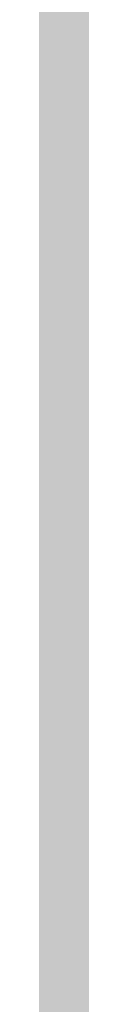
# Model space of a CAD drawing. Units: inches. Extents: x 2083 to 3317, y 1141 to 2115.
# Tile 169 of 256: x 3126.959398 to 3126.959687, y 1263.265937 to 1263.274018. Entities that reach past the tile are written whole.
import ezdxf

# ---------------------------------------------------------------- set-up
doc = ezdxf.new("R2010")
doc.units = ezdxf.units.IN
doc.layers.add('A-ANNO-DIMS', color=2, linetype='Continuous', lineweight=18)
doc.layers.add('A-WALL-PATT', color=251, linetype='Continuous', lineweight=13, true_color=0x636466)
doc.styles.get("Standard").update_dxf_attribs({"font": 'arial.ttf'})
doc.dimstyles.new('ISO-25', dxfattribs={"dimtxt": 12, "dimasz": 12, "dimexe": 1.25, "dimexo": 0.625, "dimtad": 1, "dimlunit": 3, "dimtxsty": 'Standard', "dimcen": 2.5, "dimadec": 0, "dimazin": 0, "dimtfac": 1, "dimtmove": 0, "dimatfit": 3, "dimfxl": 1, "dimarcsym": 0})

# ---------------------------------------------------------------- blocks, each defined once
blk = doc.blocks.new('*D26')
at = {"layer": 'A-ANNO-DIMS', "color": 0, "lineweight": -2, "transparency": 16777216}
for p, q in [((3088.985844, 1274.915092), (3088.985844, 1270.9519631)), ((3111.2400366, 1274.915092), (3111.2400366, 1270.9519631)), ((3076.985844, 1272.2019631), (2840.262447, 1272.2019631)), ((3111.2400366, 1272.2019631), (3088.985844, 1272.2019631)), ((3123.2400366, 1272.2019631), (3135.2400366, 1272.2019631))]:
    blk.add_line(p, q, dxfattribs=at)
at = {"layer": 'A-ANNO-DIMS', "color": 0, "transparency": 16777216}
for points in [[(3076.985844, 1274.2019631), (3076.985844, 1270.2019631), (3088.985844, 1272.2019631)], [(3123.2400366, 1274.2019631), (3123.2400366, 1270.2019631), (3111.2400366, 1272.2019631)]]:
    blk.add_solid(points, dxfattribs=at)
at = {"layer": 'Defpoints', "color": 0, "transparency": 16777216}
for p in [(3088.985844, 1275.540092), (3111.2400366, 1275.540092), (3088.985844, 1272.2019631)]:
    blk.add_point(p, dxfattribs=at)
at = {"layer": 'A-ANNO-DIMS', "color": 0, "transparency": 16777216, "insert": (2952.6241455, 1279.0316016), "char_height": 12, "attachment_point": 5}
blk.add_mtext('NIGHTSTAND 1\'-10 1/2" TYP.', dxfattribs=at)

msp = doc.modelspace()

# ---------------------------------------------------------------- hatches: boundary and pattern name
at = {"layer": 'A-WALL-PATT'}
h = msp.add_hatch(color=256, dxfattribs=at)
h.dxf.hatch_style = 1
h.paths.add_polyline_path([(3126.9597832, 2020.7613601), (2748.9597832, 2020.7613601), (2604.9597832, 2020.7613601), (2226.9597832, 2020.7613601), (2226.9597832, 1702.7613601), (2466.9597832, 1702.7613601), (2466.9597832, 1582.7613601), (2418.9597832, 1582.7613601), (2418.9597832, 1477.7613601), (2226.9597832, 1477.7613601), (2226.9597832, 1263.2613601), (2544.9597832, 1263.2613601), (2544.9597832, 1411.7613601), (2604.9597832, 1411.7613601), (2685.9597832, 1411.7613601), (2685.9597832, 1420.7613601), (2604.9597832, 1420.7613601), (2604.9597832, 1573.7613601), (2604.9597832, 1702.7613601), (2604.9597832, 2011.7613601), (2748.9597832, 2011.7613601), (2748.9597832, 1702.7613601), (2862.9597832, 1702.7613601), (2862.9597832, 1621.7613601), (2871.9597832, 1621.7613601), (2871.9597832, 1702.7613601), (2883.9597832, 1702.7613601), (2883.9597832, 1706.9394595, -0.026459), (2883.9597832, 1711.7613601), (2757.9597832, 1711.7613601), (2757.9597832, 1807.7613601), (2787.9597832, 1807.7613601), (2787.9597832, 1812.2613601), (2757.9597832, 1812.2613601), (2757.9597832, 2011.7613601), (2877.9597832, 2011.7613601), (2877.9597832, 1812.2613601), (2847.9597832, 1812.2613601), (2847.9597832, 1807.7613601), (2889.8357425, 1807.7613601), (2889.8357425, 1812.2613601), (2882.4597832, 1812.2613601), (2882.4597832, 2011.7613601), (3117.9597832, 2011.7613601), (3117.9597832, 1812.2613601), (2937.8357425, 1812.2613601), (2937.8357425, 1807.7613601), (2995.7097832, 1807.7613601), (2995.7097832, 1796.1176655), (3000.2097832, 1796.1176655), (3000.2097832, 1807.7613601), (3117.9597832, 1807.7613601), (3117.9597832, 1711.7613601), (3000.2097832, 1711.7613601), (3000.2097832, 1760.1176655), (2998.5727047, 1760.1176655, -0.020711), (2995.7097832, 1760.1176655), (2995.7097832, 1711.7613601), (2931.9597832, 1711.7613601), (2931.9597832, 1702.7613601), (3126.9597832, 1702.7613601)])
h.paths.add_polyline_path([(2471.4597832, 2011.7613601), (2471.4597832, 1810.0113601), (2462.7169357, 1810.0113601), (2462.7169357, 1805.5113601), (2505.9597832, 1805.5113601), (2505.9597832, 1810.0113601), (2475.9597832, 1810.0113601), (2475.9597832, 2011.7613601), (2595.9597832, 2011.7613601), (2595.9597832, 1810.0113601), (2565.9597832, 1810.0113601), (2565.9597832, 1805.5113601), (2595.9597832, 1805.5113601), (2595.9597832, 1711.7613601), (2235.9597832, 1711.7613601), (2235.9597832, 1805.5113601), (2353.7097832, 1805.5113601), (2353.7097832, 1796.0541624), (2358.2097832, 1796.0541624), (2358.2097832, 1805.5113601), (2414.7169357, 1805.5113601), (2414.7169357, 1810.0113601), (2235.9597832, 1810.0113601), (2235.9597832, 2011.7613601)], flags=16)
h.paths.add_polyline_path([(2270.2047343, 1994.6100082), (2270.2047343, 1970.6100082), (2246.2047343, 1970.6100082), (2246.2047343, 1994.6100082)], flags=0)
edge = h.paths.add_edge_path(flags=0)
edge.add_ellipse((2332.027391, 1899.7981761), major_axis=(-3.0429938, 3.0429938), ratio=0.16825245, start_angle=-161.3321656, end_angle=-156.3071136, ccw=False)
edge.add_ellipse((2333.0820373, 1898.7435297), major_axis=(-1.0546463, 1.0546463), ratio=0.453532097, start_angle=-123.371019, end_angle=-94.1591066)
edge = h.paths.add_edge_path(flags=0)
edge.add_ellipse((2332.027391, 1968.8762897), major_axis=(3.0429938, 3.0429938), ratio=0.16825245, start_angle=18.6678344, end_angle=23.6928864)
edge.add_spline(control_points=[(2332.9255964, 1970.6911045), (2332.2267681, 1970.3360997), (2330.8937087, 1969.6589054), (2328.4130803, 1970.9321376), (2327.2039345, 1967.7487119), (2324.7095965, 1969.9555886), (2322.5328223, 1967.012354), (2320.0128462, 1971.2958124), (2317.6803077, 1968.1578449), (2316.0405263, 1967.1020468), (2315.4269045, 1966.8096022)], knot_values=[0, 0, 0, 0, 2.267059, 4.324559, 6.685584, 8.878641, 11.121502, 14.300359, 17.755284, 19.732645, 19.732645, 19.732645, 19.732645], degree=3, periodic=0)
edge.add_ellipse((2332.027391, 1968.8762897), major_axis=(3.0429938, 3.0429938), ratio=0.16825245, start_angle=18.6678344, end_angle=23.6928864, ccw=False)
edge.add_ellipse((2333.0820373, 1969.930936), major_axis=(1.0546463, 1.0546463), ratio=0.453532097, start_angle=56.628981, end_angle=85.8408934, ccw=False)
edge = h.paths.add_edge_path(flags=0)
edge.add_spline(control_points=[(2296.4282874, 1967.9879081), (2293.6278045, 1965.3363137), (2287.7036238, 1959.727094), (2299.7438601, 1949.9956993), (2294.5325909, 1935.6685275), (2290.5732281, 1920.6035119), (2293.3941244, 1909.9736911), (2296.1854073, 1904.9665431)], knot_values=[0.099185, 0.099185, 0.099185, 0.099185, 0.345301, 0.619822, 0.982653, 1.386093, 1.810555, 1.810555, 1.810555, 1.810555], degree=3, periodic=0)
edge.add_spline(control_points=[(2296.1854073, 1904.9665431), (2297.3835817, 1902.6193002), (2298.0009694, 1901.9493116), (2298.5529698, 1901.4681549)], knot_values=[0.006246, 0.006246, 0.006246, 0.006246, 0.055476, 0.055476, 0.055476, 0.055476], degree=3, periodic=0)
edge.add_spline(control_points=[(2298.5529698, 1901.4681549), (2297.2586121, 1900.9232238), (2295.2252939, 1900.2321257), (2293.0602287, 1900.6142053), (2292.1014227, 1900.788415), (2292.0895776, 1900.790568)], knot_values=[0.312835, 0.312835, 0.312835, 0.312835, 0.40178, 0.474987, 0.475903, 0.475903, 0.475903, 0.475903], degree=3, periodic=0)
edge.add_arc((2292.7936464, 1904.6641088), 3.9370079, 215.4208969, 259.6981795, ccw=False)
edge.add_spline(control_points=[(2289.5853139, 1902.3823039), (2289.4766524, 1902.5350874), (2289.3684805, 1902.6880353), (2289.2608648, 1902.8411699)], knot_values=[0.102872, 0.102872, 0.102872, 0.102872, 0.116896, 0.116896, 0.116896, 0.116896], degree=3, periodic=0)
edge.add_spline(control_points=[(2289.2608648, 1902.8411699), (2288.6866042, 1902.5501922), (2287.6400477, 1902.0199025), (2285.8813368, 1901.8739536), (2283.8529717, 1901.5043521), (2281.7199871, 1899.7105375), (2278.4669913, 1899.492942), (2276.1571361, 1901.8832022), (2272.2589526, 1899.8040711), (2267.7776054, 1901.8431828), (2262.2438819, 1900.1840326), (2257.414927, 1901.7820606), (2254.318374, 1900.7261196), (2253.1782849, 1900.3373431)], knot_values=[0, 0, 0, 0, 1.907977, 3.477176, 5.261074, 7.972851, 11.680248, 13.717921, 16.939592, 22.789562, 27.502503, 33.595215, 37.145618, 37.145618, 37.145618, 37.145618], degree=3, periodic=0)
edge.add_line((2253.1782849, 1900.3373431), (2250.2442397, 1902.8411699))
edge.add_line((2250.2442397, 1902.8411699), (2250.2442397, 1965.8332959))
edge.add_line((2250.2442397, 1965.8332959), (2253.1782849, 1968.3371226))
edge.add_spline(control_points=[(2253.1782849, 1968.3371226), (2254.318374, 1967.9483462), (2257.414927, 1966.8924051), (2262.2438819, 1968.4904332), (2267.7776054, 1966.8312829), (2271.5267301, 1968.5372172), (2273.8759143, 1967.8282895), (2274.2067012, 1967.7276424)], knot_values=[0, 0, 0, 0, 0.09018, 0.244935, 0.364644, 0.513233, 0.537855, 0.537855, 0.537855, 0.537855], degree=3, periodic=0)
edge.add_arc((2274.3528869, 1963.7933495), 3.9370079, 72.0511336, 92.1279492, ccw=False)
edge.add_arc((2281.2969331, 1985.2300027), 18.5962982, 252.05113361, 288.56572166)
edge.add_arc((2292.3167172, 1956.0288805), 12.6460805, 71.02678788, 113.77821843, ccw=False)
edge = h.paths.add_edge_path(flags=0)
edge.add_spline(control_points=[(2274.8994147, 1951.8561946), (2275.066156, 1951.6165924), (2275.2326866, 1951.3765878), (2275.3979871, 1951.1358545)], knot_values=[1.409916, 1.409916, 1.409916, 1.409916, 1.43159, 1.43159, 1.43159, 1.43159], degree=3, periodic=0)
edge.add_spline(control_points=[(2275.3979871, 1951.1358545), (2275.7921055, 1950.5618854), (2276.1792311, 1949.9837745), (2276.5455462, 1949.3971029)], knot_values=[1.358238, 1.358238, 1.358238, 1.358238, 1.409916, 1.409916, 1.409916, 1.409916], degree=3, periodic=0)
edge.add_line((2276.5455462, 1949.3971029), (2277.437289, 1947.8621847))
edge.add_spline(control_points=[(2277.437289, 1947.8621847), (2276.3038341, 1945.6731147), (2274.6396979, 1942.4268817), (2274.631615, 1938.0938998), (2272.7991237, 1930.8515498), (2274.3564261, 1943.8970461), (2275.9476814, 1947.9233558), (2276.5455462, 1949.3971029)], knot_values=[0.005632, 0.005632, 0.005632, 0.005632, 0.186014, 0.266002, 0.357087, 0.59639, 0.739732, 0.739732, 0.739732, 0.739732], degree=3, periodic=0)
edge.add_spline(control_points=[(2276.5455462, 1949.3971029), (2276.1792311, 1949.9837745), (2275.7921055, 1950.5618854), (2275.3979871, 1951.1358545)], knot_values=[1.358238, 1.358238, 1.358238, 1.358238, 1.409916, 1.409916, 1.409916, 1.409916], degree=3, periodic=0)
edge.add_spline(control_points=[(2275.3979871, 1951.1358545), (2274.9425002, 1950.0804523), (2274.2077604, 1948.0252718), (2273.9346018, 1944.8514774), (2272.4685341, 1937.6274891), (2273.4662155, 1945.6964663), (2274.7006154, 1951.0594725), (2274.8994147, 1951.8561946)], knot_values=[0.104364, 0.104364, 0.104364, 0.104364, 0.189636, 0.269624, 0.36071, 0.600013, 0.644622, 0.644622, 0.644622, 0.644622], degree=3, periodic=0)
h.paths.add_polyline_path([(2269.1675139, 1963.1275729, -0.357527), (2268.170633, 1960.9763695, -0.092561), (2268.170633, 1939.4363249, -0.357527), (2269.1675139, 1937.2851215, -0.357527), (2267.0163105, 1938.2820024, -0.164785), (2254.6855813, 1938.2820024, -0.357527), (2252.5343779, 1937.2851215, -0.357527), (2253.5312587, 1939.4363249, -0.092561), (2253.5312587, 1960.9763695, -0.357527), (2252.5343779, 1963.1275729, -0.357527), (2254.6855813, 1962.130692, -0.164785), (2267.0163105, 1962.130692, -0.357527)], flags=0)
h.paths.add_polyline_path([(2248.8740679, 1967.8017998), (2248.8740679, 1957.0277095), (2249.4577833, 1957.0277095), (2249.4577833, 1911.6467562), (2248.8740679, 1911.6467562), (2248.8740679, 1900.8726659), (2246.5118632, 1900.8726659, 0.197327), (2244.1496584, 1902.4568734), (2244.1496584, 1966.2175923, 0.197327), (2246.5118632, 1967.8017998)], flags=0)
h.paths.add_polyline_path([(2269.1675139, 1931.3893442, -0.357527), (2268.170633, 1929.2381408, -0.092561), (2268.170633, 1907.6980962, -0.357527), (2269.1675139, 1905.5468928, -0.357527), (2267.0163105, 1906.5437737, -0.164785), (2254.6855813, 1906.5437737, -0.357527), (2252.5343779, 1905.5468928, -0.357527), (2253.5312587, 1907.6980962, -0.092561), (2253.5312587, 1929.2381408, -0.357527), (2252.5343779, 1931.3893442, -0.357527), (2254.6855813, 1930.3924634, -0.164785), (2267.0163105, 1930.3924634, -0.357527)], flags=0)
edge = h.paths.add_edge_path(flags=0)
edge.add_spline(control_points=[(2276.1968578, 1906.7237016), (2276.1681442, 1909.0289278), (2276.1140492, 1913.371852), (2270.5984171, 1924.9249783), (2273.9051746, 1919.0127787), (2275.9217115, 1916.2620626), (2275.4745699, 1912.4021495), (2277.2578735, 1910.3806206), (2276.6960436, 1908.2250358), (2276.6462176, 1906.8130226), (2276.6178249, 1906.0084068)], knot_values=[0, 0, 0, 0, 8.61026, 16.221274, 18.843057, 23.804898, 27.440828, 29.356102, 31.203478, 33.650687, 33.650687, 33.650687, 33.650687], degree=3, periodic=0)
edge.add_spline(control_points=[(2276.6178249, 1906.0084068), (2276.6233131, 1905.6241436), (2276.4977381, 1904.6286608), (2275.4417789, 1903.8547251), (2274.9373144, 1903.0804497), (2274.8590804, 1902.8411699)], knot_values=[0.156488, 0.156488, 0.156488, 0.156488, 0.184398, 0.231376, 0.250598, 0.250598, 0.250598, 0.250598], degree=3, periodic=0)
edge.add_line((2274.8590804, 1902.8411699), (2276.50598, 1902.8411699))
edge.add_spline(control_points=[(2276.50598, 1902.8411699), (2276.7883084, 1903.0849395), (2277.6650711, 1904.1251958), (2278.2495378, 1904.340738), (2277.6538719, 1908.5273866), (2278.15567, 1906.2278078), (2278.100464, 1905.2859484), (2278.8466748, 1904.0690054), (2277.8567853, 1903.4149482), (2277.8741909, 1902.9910497), (2277.9035616, 1902.8411699)], knot_values=[0.059574, 0.059574, 0.059574, 0.059574, 0.080753, 0.103741, 0.16972, 0.176036, 0.207137, 0.240474, 0.262341, 0.27366, 0.27366, 0.27366, 0.27366], degree=3, periodic=0)
edge.add_line((2277.9035616, 1902.8411699), (2280.0298255, 1902.8411699))
edge.add_spline(control_points=[(2280.0298255, 1902.8411699), (2279.8882214, 1903.088398), (2279.4992571, 1903.9815512), (2280.1522839, 1905.9393491), (2278.103615, 1909.6577572), (2279.7623946, 1907.185285), (2280.3279002, 1904.8748608), (2280.4851086, 1903.4895904), (2281.4632687, 1903.2494323), (2281.7583431, 1902.9364967), (2281.8340361, 1902.8411699)], knot_values=[0.013856, 0.013856, 0.013856, 0.013856, 0.034874, 0.088867, 0.107879, 0.126738, 0.158714, 0.193757, 0.217487, 0.226722, 0.226722, 0.226722, 0.226722], degree=3, periodic=0)
edge.add_spline(control_points=[(2281.8340361, 1902.8411699), (2281.7875348, 1902.8267029), (2281.6470224, 1902.7829881), (2281.3955272, 1902.85949), (2281.088077, 1902.9852418), (2280.7206826, 1903.060902), (2280.3334513, 1903.0257257), (2280.1247668, 1902.898879), (2280.0298255, 1902.8411699)], knot_values=[0, 0, 0, 0, 0.14413, 0.435517, 0.749276, 1.153046, 1.548371, 1.878348, 1.878348, 1.878348, 1.878348], degree=3, periodic=0)
edge.add_line((2280.0298255, 1902.8411699), (2277.9035616, 1902.8411699))
edge.add_spline(control_points=[(2277.9035616, 1902.8411699), (2277.892855, 1902.7958553), (2277.865396, 1902.6796374), (2277.6074793, 1902.6874828), (2277.2740503, 1902.8006999), (2276.8379209, 1902.6197745), (2276.5838074, 1902.7892611), (2276.50598, 1902.8411699)], knot_values=[0, 0, 0, 0, 0.127189, 0.326199, 0.628009, 1.24357, 1.515331, 1.515331, 1.515331, 1.515331], degree=3, periodic=0)
edge.add_line((2276.50598, 1902.8411699), (2274.8590804, 1902.8411699))
edge.add_spline(control_points=[(2274.8590804, 1902.8411699), (2274.8144367, 1902.8985868), (2274.7251297, 1903.013446), (2274.4934765, 1903.1189684), (2274.2442854, 1902.9605386), (2273.9371207, 1903.1849416), (2273.6140395, 1902.9831428), (2273.4083164, 1902.8830449), (2273.322254, 1902.8411699)], knot_values=[0, 0, 0, 0, 0.21843, 0.436957, 0.687977, 0.990379, 1.398396, 1.69185, 1.69185, 1.69185, 1.69185], degree=3, periodic=0)
edge.add_spline(control_points=[(2273.322254, 1902.8411699), (2273.6167403, 1903.445692), (2274.2739977, 1904.5382529), (2276.0272387, 1904.5737017), (2276.2069634, 1906.5836372), (2276.1968578, 1906.7237016)], knot_values=[0.012227, 0.012227, 0.012227, 0.012227, 0.059472, 0.106218, 0.134458, 0.134458, 0.134458, 0.134458], degree=3, periodic=0)
h.paths.add_polyline_path([(2270.7760538, 1897.7898284), (2270.7760538, 1873.7898284), (2246.7760538, 1873.7898284), (2246.7760538, 1897.7898284)], flags=0)
h.paths.add_polyline_path([(2353.7097832, 1760.0050593), (2353.7097832, 1760.0541624), (2358.2097832, 1760.0541624, -0.033729)], flags=0)
h.paths.add_polyline_path([(2321.8191188, 1737.5291862), (2341.9953271, 1737.5291862, -0.414214), (2343.2032727, 1736.3212406), (2343.2032727, 1721.0205964, -0.414214), (2341.9953271, 1719.8126508), (2321.8191188, 1719.8126508, -0.414214), (2320.6111732, 1721.0205964), (2320.6111732, 1736.3212406, -0.414214)], flags=0)
h.paths.add_polyline_path([(2324.2350099, 1736.3212406), (2339.5794359, 1736.3212406, -0.414214), (2341.9953271, 1733.9053494), (2341.9953271, 1725.4497302, -0.414214), (2339.5794359, 1723.033839), (2333.6805885, 1723.033839), (2333.8453172, 1722.0454666, -0.870646), (2335.4253988, 1721.8258934, -0.767327), (2333.922694, 1721.4232449), (2331.2910241, 1721.4232449, -0.767327), (2329.7883193, 1721.8258934, -0.870646), (2331.3684009, 1722.0454666), (2331.5331296, 1723.033839), (2324.2350099, 1723.033839, -0.414214), (2321.8191188, 1725.4497302), (2321.8191188, 1733.9053494, -0.414214)], flags=0)
h.paths.add_polyline_path([(2570.4837892, 1928.6154443), (2589.6837892, 1928.6154443), (2590.1688286, 1928.6154443), (2590.1688286, 1904.9933971), (2570.4837892, 1904.9933971)], flags=0)
h.paths.add_polyline_path([(2574.4473242, 1927.2638215, -1), (2572.8288357, 1927.2638215, -1)], flags=0)
h.paths.add_polyline_path([(2573.0898665, 1926.9408768), (2573.925032, 1927.7760423), (2574.1477428, 1927.5533315), (2573.3125773, 1926.718166)], flags=0)
h.paths.add_polyline_path([(2578.7790648, 1919.7296175, -1), (2571.5916632, 1919.7296175, -1)], flags=0)
h.paths.add_polyline_path([(2578.385364, 1919.7296175, -1), (2571.985364, 1919.7296175, -1)], flags=0)
h.paths.add_polyline_path([(2331.5957638, 1729.4762156, -1), (2333.6179542, 1729.4762156, -1)], flags=0)
h.paths.add_polyline_path([(2578.0342282, 1927.2638215, -1), (2576.4157396, 1927.2638215, -1)], flags=0)
h.paths.add_polyline_path([(2576.6888513, 1927.5310886), (2576.9115621, 1927.7537993), (2577.7467276, 1926.9186339), (2577.5240168, 1926.6959231)], flags=0)
h.paths.add_polyline_path([(2578.1390648, 1909.8595388, -1), (2572.2316632, 1909.8595388, -1)], flags=0)
h.paths.add_polyline_path([(2577.745364, 1909.8595388, -1), (2572.625364, 1909.8595388, -1)], flags=0)
h.paths.add_polyline_path([(2583.7977179, 1927.2638215, -1), (2582.1792294, 1927.2638215, -1)], flags=0)
h.paths.add_polyline_path([(2582.7186487, 1927.7537993), (2583.5538142, 1926.9186339), (2583.3311034, 1926.6959231), (2582.4959379, 1927.5310886)], flags=0)
h.paths.add_polyline_path([(2582.4959379, 1927.5310886), (2582.7186487, 1927.7537993), (2583.5538142, 1926.9186339), (2583.3311034, 1926.6959231)], flags=0)
h.paths.add_polyline_path([(2587.7390648, 1920.5296175, -1), (2581.8316632, 1920.5296175, -1)], flags=0)
h.paths.add_polyline_path([(2587.345364, 1920.5296175, -1), (2582.225364, 1920.5296175, -1)], flags=0)
h.paths.add_polyline_path([(2587.3846219, 1927.2638215, -1), (2585.7661333, 1927.2638215, -1)], flags=0)
h.paths.add_polyline_path([(2586.0819925, 1926.9802469), (2586.917158, 1927.8154124), (2587.1398688, 1927.5927016), (2586.3047033, 1926.7575361)], flags=0)
h.paths.add_polyline_path([(2588.3790648, 1910.6595388, -1), (2581.1916632, 1910.6595388, -1)], flags=0)
h.paths.add_polyline_path([(2587.985364, 1910.6595388, -1), (2581.585364, 1910.6595388, -1)], flags=0)
h.paths.add_polyline_path([(2417.1677288, 1729.4778955), (2437.3439372, 1729.4778955, -0.414214), (2438.5518828, 1728.2699499), (2438.5518828, 1712.9693057, -0.414214), (2437.3439372, 1711.7613601), (2417.1677288, 1711.7613601, -0.414214), (2415.9597832, 1712.9693057), (2415.9597832, 1728.2699499, -0.414214)], flags=0)
h.paths.add_polyline_path([(2419.58362, 1728.2699499), (2434.928046, 1728.2699499, -0.414214), (2437.3439372, 1725.8540587), (2437.3439372, 1717.3984395, -0.414214), (2434.928046, 1714.9825483), (2429.0291985, 1714.9825483), (2429.1939273, 1713.9941758, -0.870646), (2430.7740089, 1713.7746027, -0.767327), (2429.2713041, 1713.3719542), (2426.6396342, 1713.3719542, -0.767327), (2425.1369294, 1713.7746027, -0.870646), (2426.717011, 1713.9941758), (2426.8817397, 1714.9825483), (2419.58362, 1714.9825483, -0.414214), (2417.1677288, 1717.3984395), (2417.1677288, 1725.8540587, -0.414214)], flags=0)
h.paths.add_polyline_path([(2419.58362, 1728.2699499), (2434.928046, 1728.2699499, -0.414214), (2437.3439372, 1725.8540587), (2437.3439372, 1717.3984395, -0.414214), (2434.928046, 1714.9825483), (2429.0291985, 1714.9825483), (2428.3581177, 1719.0090337), (2427.5528206, 1719.0090337), (2426.8817397, 1714.9825483), (2419.58362, 1714.9825483, -0.414214), (2417.1677288, 1717.3984395), (2417.1677288, 1725.8540587, -0.414214)], flags=0)
h.paths.add_polyline_path([(2426.9443739, 1721.4249248, -1), (2428.9665643, 1721.4249248, -1)], flags=0)
h.paths.add_polyline_path([(2475.9597832, 1702.7613601), (2595.9597832, 1702.7613601), (2595.9597832, 1582.7613601), (2475.9597832, 1582.7613601)], flags=16)
h.paths.add_polyline_path([(2427.9597832, 1573.7613601), (2595.9597832, 1573.7613601), (2595.9597832, 1468.7613601), (2595.9597832, 1420.7613601), (2384.4597832, 1420.7613601), (2384.4597832, 1468.7613601), (2427.9597832, 1468.7613601)], flags=16)
h.paths.add_polyline_path([(2379.9597832, 1468.7613601), (2379.9597832, 1420.7613601), (2235.9597832, 1420.7613601), (2235.9597832, 1468.7613601)], flags=16)
h.paths.add_polyline_path([(2317.8159962, 1466.695767), (2337.9922045, 1466.695767, -0.414214), (2339.2001501, 1465.4878214), (2339.2001501, 1450.1871771, -0.414214), (2337.9922045, 1448.9792315), (2317.8159962, 1448.9792315, -0.414214), (2316.6080506, 1450.1871771), (2316.6080506, 1465.4878214, -0.414214)], flags=0)
h.paths.add_polyline_path([(2320.2318874, 1465.4878214), (2335.5763133, 1465.4878214, -0.414214), (2337.9922045, 1463.0719302), (2337.9922045, 1454.616311, -0.414214), (2335.5763133, 1452.2004198), (2329.6774659, 1452.2004198), (2329.8421946, 1451.2120473, -0.870646), (2331.4222762, 1450.9924742, -0.767327), (2329.9195714, 1450.5898257), (2327.2879015, 1450.5898257, -0.767327), (2325.7851967, 1450.9924742, -0.870646), (2327.3652783, 1451.2120473), (2327.530007, 1452.2004198), (2320.2318874, 1452.2004198, -0.414214), (2317.8159962, 1454.616311), (2317.8159962, 1463.0719302, -0.414214)], flags=0)
h.paths.add_polyline_path([(2320.2318874, 1465.4878214), (2335.5763133, 1465.4878214, -0.414214), (2337.9922045, 1463.0719302), (2337.9922045, 1454.616311, -0.414214), (2335.5763133, 1452.2004198), (2329.6774659, 1452.2004198), (2329.006385, 1456.2269051), (2328.2010879, 1456.2269051), (2327.530007, 1452.2004198), (2320.2318874, 1452.2004198, -0.414214), (2317.8159962, 1454.616311), (2317.8159962, 1463.0719302, -0.414214)], flags=0)
h.paths.add_polyline_path([(2327.5926413, 1458.6427963, -1), (2329.6148317, 1458.6427963, -1)], flags=0)
h.paths.add_polyline_path([(2244.4117436, 1433.3404531), (2241.9209449, 1433.3404531, -0.414214), (2240.0178562, 1435.2435418), (2240.0178562, 1440.9528078, -0.414211), (2241.920925, 1442.8558965), (2244.4117436, 1442.8558965, -1.976472)], flags=0)
h.paths.add_polyline_path([(2245.3568884, 1434.3975358, -0.414214), (2245.3568884, 1441.7988138, -2.144098)], flags=0)
h.paths.add_polyline_path([(2535.9597832, 1416.2613601), (2535.9597832, 1272.2613601), (2235.9597832, 1272.2613601), (2235.9597832, 1416.2613601)], flags=16)
h.paths.add_polyline_path([(2260.1195614, 1384.2928413), (2260.1195614, 1362.0386487), (2237.8653688, 1362.0386487), (2237.8653688, 1384.2928413)], flags=0)
edge = h.paths.add_edge_path(flags=0)
edge.add_line((2318.2518466, 1362.0932983), (2318.1457968, 1362.0009726))
edge.add_ellipse((2317.4451158, 1360.4310442), major_axis=(2.8216404, 2.8216404), ratio=0.16825245, start_angle=18.6678344, end_angle=20.9481273, ccw=False)
edge.add_ellipse((2318.4230451, 1361.4089735), major_axis=(0.9779293, 0.9779293), ratio=0.453532097, start_angle=56.628981, end_angle=70.2262012, ccw=False)
edge = h.paths.add_edge_path(flags=0)
edge.add_line((2319.1073699, 1295.5710784), (2319.0150442, 1295.6771282))
edge.add_ellipse((2317.4451158, 1296.3778091), major_axis=(-2.8216404, 2.8216404), ratio=0.16825245, start_angle=-161.3321656, end_angle=-159.0518727, ccw=False)
edge.add_ellipse((2318.4230451, 1295.3998798), major_axis=(-0.9779293, 0.9779293), ratio=0.453532097, start_angle=-123.371019, end_angle=-109.7737988)
edge = h.paths.add_edge_path(flags=0)
edge.add_spline(control_points=[(2284.2103489, 1301.1702189), (2284.5806878, 1300.444719), (2284.8911891, 1299.8920243), (2285.159553, 1299.4610182)], knot_values=[0.039066, 0.039066, 0.039066, 0.039066, 0.055476, 0.055476, 0.055476, 0.055476], degree=3, periodic=0)
edge.add_line((2285.159553, 1299.4610182), (2284.2103489, 1301.1702189))
edge = h.paths.add_edge_path(flags=0)
edge.add_line((2280.4124579, 1297.2980125), (2283.3699905, 1297.0361216))
edge.add_line((2283.3699905, 1297.0361216), (2286.4056902, 1297.9263104))
edge.add_spline(control_points=[(2286.4056902, 1297.9263104), (2285.305487, 1297.4631193), (2284.3447774, 1297.1291508), (2283.3699905, 1297.0361216)], knot_values=[0.394369, 0.394369, 0.394369, 0.394369, 0.475903, 0.475903, 0.475903, 0.475903], degree=3, periodic=0)
edge.add_spline(control_points=[(2283.3699905, 1297.0361216), (2283.2813895, 1297.027666), (2282.316289, 1296.9573356), (2281.3125019, 1297.1344787), (2280.4234414, 1297.2960161), (2280.4124579, 1297.2980125)], knot_values=[0.312835, 0.312835, 0.312835, 0.312835, 0.320246, 0.393453, 0.394369, 0.394369, 0.394369, 0.394369], degree=3, periodic=0)
edge = h.paths.add_edge_path(flags=0)
edge.add_line((2284.4355615, 1359.6072854), (2280.4462909, 1355.328047))
edge.add_line((2280.4462909, 1355.328047), (2279.5799868, 1351.0177544))
edge.add_line((2279.5799868, 1351.0177544), (2282.4129737, 1346.5804327))
edge.add_spline(control_points=[(2282.4129737, 1346.5804327), (2283.1533308, 1345.5892358), (2284.2528957, 1344.0288973), (2284.801037, 1342.3871671), (2284.9351625, 1341.8055443)], knot_values=[1.240098, 1.240098, 1.240098, 1.240098, 1.332892, 1.382712, 1.382712, 1.382712, 1.382712], degree=3, periodic=0)
edge.add_spline(control_points=[(2284.9351625, 1341.8055443), (2285.3191079, 1340.1406002), (2285.2330291, 1338.4092041), (2284.9099384, 1336.6541222)], knot_values=[1.097484, 1.097484, 1.097484, 1.097484, 1.240098, 1.240098, 1.240098, 1.240098], degree=3, periodic=0)
edge.add_spline(control_points=[(2284.9099384, 1336.6541222), (2284.5868478, 1334.8990403), (2284.0267453, 1333.1202725), (2283.4626437, 1331.3605849)], knot_values=[0.95487, 0.95487, 0.95487, 0.95487, 1.097484, 1.097484, 1.097484, 1.097484], degree=3, periodic=0)
edge.add_line((2283.4626437, 1331.3605849), (2281.8903759, 1326.153357))
edge.add_line((2281.8903759, 1326.153357), (2280.7562592, 1321.0560888))
edge.add_line((2280.7562592, 1321.0560888), (2280.2992048, 1316.0019772))
edge.add_line((2280.2992048, 1316.0019772), (2280.7159327, 1310.9500678))
edge.add_line((2280.7159327, 1310.9500678), (2282.0280939, 1305.9721367))
edge.add_line((2282.0280939, 1305.9721367), (2284.2103489, 1301.1702189))
edge.add_spline(control_points=[(2284.2103489, 1301.1702189), (2283.3407305, 1302.7301854), (2282.6119044, 1304.3364933), (2282.0280939, 1305.9721367)], knot_values=[0.099185, 0.099185, 0.099185, 0.099185, 0.241799, 0.241799, 0.241799, 0.241799], degree=3, periodic=0)
edge.add_spline(control_points=[(2282.0280939, 1305.9721367), (2281.4442835, 1307.6077801), (2281.0054886, 1309.2727591), (2280.7159327, 1310.9500678)], knot_values=[0.241799, 0.241799, 0.241799, 0.241799, 0.384413, 0.384413, 0.384413, 0.384413], degree=3, periodic=0)
edge.add_spline(control_points=[(2280.7159327, 1310.9500678), (2280.4332411, 1312.5876134), (2280.2893863, 1314.2769594), (2280.2988938, 1315.9620324), (2280.2992048, 1316.0019772)], knot_values=[0.384413, 0.384413, 0.384413, 0.384413, 0.523647, 0.527028, 0.527028, 0.527028, 0.527028], degree=3, periodic=0)
edge.add_spline(control_points=[(2280.2992048, 1316.0019772), (2280.3123257, 1317.6869552), (2280.4778706, 1319.3679256), (2280.7562592, 1321.0560888)], knot_values=[0.527028, 0.527028, 0.527028, 0.527028, 0.669642, 0.669642, 0.669642, 0.669642], degree=3, periodic=0)
edge.add_spline(control_points=[(2280.7562592, 1321.0560888), (2281.0346478, 1322.7442519), (2281.4258801, 1324.4396079), (2281.8903759, 1326.153357)], knot_values=[0.669642, 0.669642, 0.669642, 0.669642, 0.812256, 0.812256, 0.812256, 0.812256], degree=3, periodic=0)
edge.add_spline(control_points=[(2281.8903759, 1326.153357), (2282.2643834, 1327.5332507), (2282.7878702, 1329.2618097), (2283.352751, 1331.0177803), (2283.4626437, 1331.3605849)], knot_values=[0.812256, 0.812256, 0.812256, 0.812256, 0.927087, 0.95487, 0.95487, 0.95487, 0.95487], degree=3, periodic=0)
edge.add_line((2283.4626437, 1331.3605849), (2284.9099384, 1336.6541222))
edge.add_line((2284.9099384, 1336.6541222), (2284.9351625, 1341.8055443))
edge.add_line((2284.9351625, 1341.8055443), (2282.4129737, 1346.5804327))
edge.add_spline(control_points=[(2282.4129737, 1346.5804327), (2281.2751273, 1348.1037918), (2280.0784467, 1349.5703178), (2279.5799868, 1351.0177544)], knot_values=[1.382712, 1.382712, 1.382712, 1.382712, 1.525326, 1.525326, 1.525326, 1.525326], degree=3, periodic=0)
edge.add_spline(control_points=[(2279.5799868, 1351.0177544), (2279.4432818, 1351.4147209), (2279.1363124, 1352.856922), (2279.7351897, 1354.2903851), (2280.4462909, 1355.328047)], knot_values=[1.525326, 1.525326, 1.525326, 1.525326, 1.564439, 1.667941, 1.667941, 1.667941, 1.667941], degree=3, periodic=0)
edge.add_spline(control_points=[(2280.4462909, 1355.328047), (2281.4261132, 1356.7578354), (2282.9308373, 1358.1825604), (2284.4355615, 1359.6072854)], knot_values=[1.667941, 1.667941, 1.667941, 1.667941, 1.810555, 1.810555, 1.810555, 1.810555], degree=3, periodic=0)
edge.add_arc((2280.6230749, 1348.518181), 11.7261796, 71.02678788, 113.77821843)
edge.add_arc((2270.4048917, 1375.5951559), 17.2435667, 252.05113361, 288.56572166, ccw=False)
edge.add_arc((2263.9659692, 1355.7178471), 3.6506221, 72.0511336, 92.1279492)
edge.add_arc((2263.9659692, 1355.7178471), 3.6506221, 92.1279492, 177.98513)
edge.add_spline(control_points=[(2260.3176041, 1355.8461989), (2260.2604169, 1354.2206683), (2260.551278, 1350.1865469), (2262.9993445, 1346.7662507), (2264.4727415, 1344.6490245)], knot_values=[1.43159, 1.43159, 1.43159, 1.43159, 1.564144, 1.770695, 1.770695, 1.770695, 1.770695], degree=3, periodic=0)
edge.add_line((2264.4727415, 1344.6490245), (2264.9355904, 1343.9825301))
edge.add_spline(control_points=[(2263.8010444, 1340.2481052), (2263.8432379, 1340.5140884), (2264.0672444, 1341.7564652), (2264.5126928, 1343.0024532), (2264.9350468, 1343.9810834)], knot_values=[0.53657, 0.53657, 0.53657, 0.53657, 0.559349, 0.644622, 0.644622, 0.644622, 0.644622], degree=3, periodic=0)
edge.add_spline(control_points=[(2264.9350468, 1343.9810834), (2265.1177715, 1343.7149747), (2265.2988751, 1343.4479058), (2265.4767562, 1343.1793646)], knot_values=[1.384077, 1.384077, 1.384077, 1.384077, 1.409916, 1.409916, 1.409916, 1.409916], degree=3, periodic=0)
edge.add_spline(control_points=[(2265.4767562, 1343.1793646), (2265.6546373, 1342.9108234), (2265.8292958, 1342.64081), (2265.9991301, 1342.368812)], knot_values=[1.358238, 1.358238, 1.358238, 1.358238, 1.384077, 1.384077, 1.384077, 1.384077], degree=3, periodic=0)
edge.add_line((2265.9991301, 1342.368812), (2266.8260057, 1340.9455468))
edge.add_spline(control_points=[(2266.8260057, 1340.9455468), (2268.894401, 1337.0896912), (2271.3981727, 1325.8430009), (2270.5161644, 1310.5685568), (2275.9193759, 1301.860609), (2277.7895113, 1299.1994495)], knot_values=[0.116896, 0.116896, 0.116896, 0.116896, 0.472987, 1.050969, 1.313793, 1.313793, 1.313793, 1.313793], degree=3, periodic=0)
edge.add_spline(control_points=[(2277.7895113, 1299.1994495), (2277.8394051, 1299.1284519), (2277.8894277, 1299.0574975), (2277.9395717, 1298.9865839)], knot_values=[0.109884, 0.109884, 0.109884, 0.109884, 0.116896, 0.116896, 0.116896, 0.116896], degree=3, periodic=0)
edge.add_line((2277.9395717, 1298.9865839), (2277.7888489, 1299.1991139))
edge.add_spline(control_points=[(2277.7888489, 1299.1991139), (2277.2565819, 1298.9294144), (2276.2863504, 1298.4379024), (2275.0393517, 1298.3344186), (2274.3833299, 1298.2388951), (2274.2152543, 1298.209338)], knot_values=[33.12187, 33.12187, 33.12187, 33.12187, 35.029056, 36.598255, 37.144827, 37.144827, 37.144827, 37.144827], degree=3, periodic=0)
edge.add_line((2274.2152543, 1298.209338), (2273.073147, 1297.8929607))
edge.add_spline(control_points=[(2273.073147, 1297.8929607), (2272.3229363, 1297.579784), (2271.0391507, 1296.5105078), (2269.2483948, 1296.2260622), (2268.4231004, 1296.3746543)], knot_values=[26.532584, 26.532584, 26.532584, 26.532584, 29.198919, 31.839101, 31.839101, 31.839101, 31.839101], degree=3, periodic=0)
edge.add_line((2268.4231004, 1296.3746543), (2263.8785014, 1297.4575338))
edge.add_spline(control_points=[(2263.8785014, 1297.4575338), (2263.5560769, 1297.3594345), (2261.8603064, 1296.8386943), (2260.2387805, 1297.2824073), (2258.9334543, 1297.5164611)], knot_values=[15.919551, 15.919551, 15.919551, 15.919551, 16.939592, 21.226067, 21.226067, 21.226067, 21.226067], degree=3, periodic=0)
edge.add_line((2258.9334543, 1297.5164611), (2254.0552332, 1297.3290098))
edge.add_spline(control_points=[(2254.0552332, 1297.3290098), (2253.7555255, 1297.295815), (2252.1136834, 1297.1651738), (2250.4618687, 1297.5442209), (2249.1296862, 1297.6678818)], knot_values=[5.306517, 5.306517, 5.306517, 5.306517, 6.276435, 10.613034, 10.613034, 10.613034, 10.613034], degree=3, periodic=0)
edge.add_line((2249.1296862, 1297.6678818), (2244.3316495, 1296.8777561))
edge.add_line((2244.3316495, 1296.8777561), (2241.6110326, 1299.1994495))
edge.add_line((2241.6110326, 1299.1994495), (2241.6110326, 1357.6094038))
edge.add_line((2241.6110326, 1357.6094038), (2244.3316495, 1359.9310973))
edge.add_line((2244.3316495, 1359.9310973), (2252.7288228, 1359.5426917))
edge.add_spline(control_points=[(2252.7288228, 1359.5426917), (2252.8709387, 1359.5464396), (2253.3057402, 1359.5481716), (2253.7398447, 1359.5142744), (2254.0317419, 1359.4824261)], knot_values=[0.233291, 0.233291, 0.233291, 0.233291, 0.244935, 0.268927, 0.268927, 0.268927, 0.268927], degree=3, periodic=0)
edge.add_line((2254.0317419, 1359.4824261), (2259.5871899, 1359.4163899))
edge.add_spline(control_points=[(2259.5871899, 1359.4163899), (2260.6770676, 1359.6285026), (2262.0731971, 1359.8970025), (2263.5236925, 1359.4592776), (2263.8304173, 1359.3659518)], knot_values=[0.422516, 0.422516, 0.422516, 0.422516, 0.513233, 0.537855, 0.537855, 0.537855, 0.537855], degree=3, periodic=0)
edge.add_arc((2263.9659692, 1355.7178471), 3.6506221, 72.0511336, 92.1279492, ccw=False)
edge.add_arc((2270.4048917, 1375.5951559), 17.2435667, 252.05113361, 288.56572166)
edge.add_arc((2280.6230749, 1348.518181), 11.7261796, 71.02678788, 113.77821843, ccw=False)
h.paths.add_polyline_path([(2240.3405298, 1359.4347149), (2240.3405298, 1349.4443532), (2240.8817846, 1349.4443532), (2240.8817846, 1307.3645001), (2240.3405298, 1307.3645001), (2240.3405298, 1297.3741385), (2238.1501565, 1297.3741385, 0.197327), (2235.9597832, 1298.8431076), (2235.9597832, 1357.9657458, 0.197327), (2238.1501565, 1359.4347149)], flags=0)
h.paths.add_polyline_path([(2259.1577904, 1355.1005005, -0.357527), (2258.2334246, 1353.1057799, -0.092561), (2258.2334246, 1333.1326007, -0.357527), (2259.1577904, 1331.1378801, -0.357527), (2257.1630698, 1332.0622458, -0.164785), (2245.7293022, 1332.0622458, -0.357527), (2243.7345816, 1331.1378801, -0.357527), (2244.6589474, 1333.1326007, -0.092561), (2244.6589474, 1353.1057799, -0.357527), (2243.7345816, 1355.1005005, -0.357527), (2245.7293022, 1354.1761347, -0.164785), (2257.1630698, 1354.1761347, -0.357527)], flags=0)
edge = h.paths.add_edge_path(flags=0)
edge.add_line((2265.9991301, 1342.368812), (2266.8260057, 1340.9455468))
edge.add_line((2266.8260057, 1340.9455468), (2265.3075567, 1337.8140664))
edge.add_line((2265.3075567, 1337.8140664), (2264.358232, 1334.6529388))
edge.add_line((2264.358232, 1334.6529388), (2264.2620123, 1333.7997046))
edge.add_spline(control_points=[(2264.2620123, 1333.7997046), (2264.2083565, 1333.187055), (2264.1620602, 1332.3655252), (2264.0071444, 1331.4139326), (2263.9690487, 1331.2018338)], knot_values=[0.464444, 0.464444, 0.464444, 0.464444, 0.516691, 0.531608, 0.531608, 0.531608, 0.531608], degree=3, periodic=0)
edge.add_spline(control_points=[(2263.9690487, 1331.2018338), (2263.7745349, 1330.1188727), (2263.4243703, 1328.7908386), (2263.2574202, 1328.5306516), (2263.2340282, 1328.5146115)], knot_values=[0.372682, 0.372682, 0.372682, 0.372682, 0.44885, 0.464444, 0.464444, 0.464444, 0.464444], degree=3, periodic=0)
edge.add_spline(control_points=[(2263.2340282, 1328.5146115), (2263.096382, 1328.4202271), (2263.1311696, 1329.3014765), (2263.2749528, 1330.6157493)], knot_values=[0.280919, 0.280919, 0.280919, 0.280919, 0.372682, 0.372682, 0.372682, 0.372682], degree=3, periodic=0)
edge.add_spline(control_points=[(2263.2749528, 1330.6157493), (2263.4187361, 1331.930022), (2263.6715151, 1333.677318), (2263.9698519, 1335.3150268)], knot_values=[0.189157, 0.189157, 0.189157, 0.189157, 0.280919, 0.280919, 0.280919, 0.280919], degree=3, periodic=0)
edge.add_spline(control_points=[(2263.9698519, 1335.3150268), (2264.1004958, 1336.0321917), (2264.4187827, 1337.6219113), (2264.7548476, 1338.8644304), (2264.9474193, 1339.4911244)], knot_values=[0.097394, 0.097394, 0.097394, 0.097394, 0.137578, 0.189157, 0.189157, 0.189157, 0.189157], degree=3, periodic=0)
edge.add_spline(control_points=[(2264.9474193, 1339.4911244), (2265.2900171, 1340.6060546), (2265.6442376, 1341.4939958), (2265.9991301, 1342.368812)], knot_values=[0.005632, 0.005632, 0.005632, 0.005632, 0.097394, 0.097394, 0.097394, 0.097394], degree=3, periodic=0)
h.paths.add_polyline_path([(2259.1577904, 1325.6709733, -0.357527), (2258.2334246, 1323.6762527, -0.092561), (2258.2334246, 1303.7030735, -0.357527), (2259.1577904, 1301.7083529, -0.357527), (2257.1630698, 1302.6327186, -0.164785), (2245.7293022, 1302.6327186, -0.357527), (2243.7345816, 1301.7083529, -0.357527), (2244.6589474, 1303.7030735, -0.092561), (2244.6589474, 1323.6762527, -0.357527), (2243.7345816, 1325.6709733, -0.357527), (2245.7293022, 1324.7466075, -0.164785), (2257.1630698, 1324.7466075, -0.357527)], flags=0)
edge = h.paths.add_edge_path(flags=0)
edge.add_spline(control_points=[(2261.7089377, 1317.3114208), (2261.6794818, 1317.4175798), (2261.7618581, 1317.3885347), (2262.4907358, 1316.0898725), (2262.962185, 1315.3008975)], knot_values=[14.955861, 14.955861, 14.955861, 14.955861, 16.221274, 18.694826, 18.694826, 18.694826, 18.694826], degree=3, periodic=0)
edge.add_spline(control_points=[(2262.962185, 1315.3008975), (2262.9904374, 1315.2536169), (2263.7020958, 1314.0673762), (2264.3489834, 1313.1271533), (2264.7300545, 1312.1641544)], knot_values=[18.694826, 18.694826, 18.694826, 18.694826, 18.843057, 22.433791, 22.433791, 22.433791, 22.433791], degree=3, periodic=0)
edge.add_spline(control_points=[(2264.7300545, 1312.1641544), (2264.8755649, 1311.7964373), (2265.1768733, 1310.7698073), (2265.1430689, 1309.5592623), (2265.2477363, 1308.8241926)], knot_values=[22.433791, 22.433791, 22.433791, 22.433791, 23.804898, 26.172756, 26.172756, 26.172756, 26.172756], degree=3, periodic=0)
edge.add_line((2265.2477363, 1308.8241926), (2265.8507741, 1307.1718879))
edge.add_spline(control_points=[(2265.8507741, 1307.1718879), (2266.0650246, 1306.8216779), (2266.3843872, 1306.3322461), (2266.4244001, 1305.7805489), (2266.4203688, 1305.6112163)], knot_values=[28.062562, 28.062562, 28.062562, 28.062562, 29.356102, 29.911721, 29.911721, 29.911721, 29.911721], degree=3, periodic=0)
edge.add_spline(control_points=[(2266.4203688, 1305.6112163), (2266.4161162, 1305.4325896), (2266.393999, 1305.2499979), (2266.3647773, 1305.0658571)], knot_values=[29.911721, 29.911721, 29.911721, 29.911721, 30.497837, 30.497837, 30.497837, 30.497837], degree=3, periodic=0)
edge.add_line((2266.3647773, 1305.0658571), (2266.0661511, 1302.1362954))
edge.add_spline(control_points=[(2266.0661511, 1302.1362954), (2266.0712401, 1301.7799843), (2265.9980761, 1301.1999847), (2265.6632664, 1300.7589613), (2265.5089084, 1300.5858824)], knot_values=[0.156488, 0.156488, 0.156488, 0.156488, 0.184398, 0.203543, 0.203543, 0.203543, 0.203543], degree=3, periodic=0)
edge.add_line((2265.5089084, 1300.5858824), (2264.4353411, 1299.1994495))
edge.add_line((2264.4353411, 1299.1994495), (2265.962442, 1299.1994495))
edge.add_line((2265.962442, 1299.1994495), (2267.3359898, 1301.1752758))
edge.add_line((2267.3359898, 1301.1752758), (2267.3116668, 1301.9862366))
edge.add_spline(control_points=[(2267.3116668, 1301.9862366), (2267.261111, 1302.8623959), (2267.1602121, 1303.7371316), (2267.2714865, 1303.3258962)], knot_values=[0.126229, 0.126229, 0.126229, 0.126229, 0.166617, 0.166617, 0.166617, 0.166617], degree=3, periodic=0)
edge.add_spline(control_points=[(2267.2714865, 1303.3258962), (2267.2800347, 1303.2943047), (2267.3097851, 1303.1753659), (2267.3734504, 1302.8836084), (2267.4061233, 1302.6828291), (2267.4179259, 1302.6010251)], knot_values=[0.166617, 0.166617, 0.166617, 0.166617, 0.16972, 0.176036, 0.180765, 0.180765, 0.180765, 0.180765], degree=3, periodic=0)
edge.add_spline(control_points=[(2267.7438914, 1300.9875045), (2267.6875832, 1301.1509426), (2267.4805198, 1301.6566644), (2267.4837514, 1302.1447877), (2267.4179259, 1302.6010251)], knot_values=[0.180765, 0.180765, 0.180765, 0.180765, 0.193767, 0.220139, 0.220139, 0.220139, 0.220139], degree=3, periodic=0)
edge.add_line((2267.4179259, 1302.6010251), (2267.7438914, 1300.9875045))
edge.add_spline(control_points=[(2267.7438914, 1300.9875045), (2267.8319608, 1300.7318778), (2267.9320205, 1300.3099042), (2267.5548409, 1299.9745185), (2267.429366, 1299.8292073)], knot_values=[0.220139, 0.220139, 0.220139, 0.220139, 0.240474, 0.25489, 0.25489, 0.25489, 0.25489], degree=3, periodic=0)
edge.add_line((2267.429366, 1299.8292073), (2267.2583608, 1299.1994495))
edge.add_line((2267.2583608, 1299.1994495), (2269.229956, 1299.1994495))
edge.add_spline(control_points=[(2269.229956, 1299.1994495), (2269.0986525, 1299.4286938), (2268.842774, 1300.0162509), (2269.0115749, 1300.9159235), (2268.9467957, 1301.6607397)], knot_values=[0.013856, 0.013856, 0.013856, 0.013856, 0.034874, 0.067073, 0.067073, 0.067073, 0.067073], degree=3, periodic=0)
edge.add_line((2268.9467957, 1301.6607397), (2268.4315815, 1303.6031089))
edge.add_spline(control_points=[(2268.4315815, 1303.6031089), (2268.1755957, 1304.1923747), (2267.5962136, 1305.2512977), (2268.0406981, 1304.6232098), (2268.2513938, 1304.2824205)], knot_values=[0.090155, 0.090155, 0.090155, 0.090155, 0.107879, 0.120289, 0.120289, 0.120289, 0.120289], degree=3, periodic=0)
edge.add_spline(control_points=[(2268.2513938, 1304.2824205), (2268.3608818, 1304.1053294), (2269.0577527, 1302.9179833), (2269.382691, 1301.5904186), (2269.5214051, 1300.7759312), (2269.5752202, 1300.5557836)], knot_values=[0.120289, 0.120289, 0.120289, 0.120289, 0.126738, 0.158714, 0.173506, 0.173506, 0.173506, 0.173506], degree=3, periodic=0)
edge.add_line((2269.5752202, 1300.5557836), (2270.6857984, 1299.4212579))
edge.add_spline(control_points=[(2270.6857984, 1299.4212579), (2270.7672206, 1299.3572512), (2270.8378523, 1299.2814011), (2270.9029248, 1299.1994495)], knot_values=[0.21816, 0.21816, 0.21816, 0.21816, 0.226722, 0.226722, 0.226722, 0.226722], degree=3, periodic=0)
edge.add_line((2270.9372012, 1299.1929131), (2270.9029248, 1299.1994495))
edge.add_spline(control_points=[(2270.9029248, 1299.1994495), (2270.8598061, 1299.1860349), (2270.7295148, 1299.1455), (2270.4963139, 1299.216437), (2270.2716612, 1299.3083234), (2270.1210168, 1299.3479612), (2270.0633386, 1299.3595566)], knot_values=[0.939174, 0.939174, 0.939174, 0.939174, 1.083304, 1.374691, 1.68845, 1.878348, 1.878348, 1.878348, 1.878348], degree=3, periodic=0)
edge.add_line((2270.0633386, 1299.3595566), (2269.229956, 1299.1994495))
edge.add_line((2269.229956, 1299.1994495), (2267.2583608, 1299.1994495))
edge.add_spline(control_points=[(2267.2583608, 1299.1994495), (2267.248433, 1299.1574312), (2267.2229714, 1299.0496673), (2266.9838161, 1299.056942), (2266.8092097, 1299.1162303), (2266.6769047, 1299.1090913), (2266.636531, 1299.1048147)], knot_values=[0.757665, 0.757665, 0.757665, 0.757665, 0.884854, 1.083864, 1.385675, 1.515331, 1.515331, 1.515331, 1.515331], degree=3, periodic=0)
edge.add_spline(control_points=[(2266.636531, 1299.1048147), (2266.4852248, 1299.0887878), (2266.2358066, 1299.0171229), (2266.0346081, 1299.1513168), (2265.962442, 1299.1994495)], knot_values=[0, 0, 0, 0, 0.485905, 0.757665, 0.757665, 0.757665, 0.757665], degree=3, periodic=0)
edge.add_line((2265.962442, 1299.1994495), (2264.4353411, 1299.1994495))
edge.add_line((2264.4353411, 1299.1994495), (2263.8584442, 1299.3671176))
edge.add_spline(control_points=[(2263.8584442, 1299.3671176), (2263.8189433, 1299.3709053), (2263.7795277, 1299.3857212), (2263.7401308, 1299.4015039)], knot_values=[0.845925, 0.845925, 0.845925, 0.845925, 0.978627, 0.978627, 0.978627, 0.978627], degree=3, periodic=0)
edge.add_line((2263.7217862, 1299.3964251), (2263.0103065, 1299.1994495))
edge.add_spline(control_points=[(2263.0103065, 1299.1994495), (2263.2457942, 1299.682859), (2263.5060317, 1300.1281072), (2263.8734943, 1300.4080279)], knot_values=[0.012227, 0.012227, 0.012227, 0.012227, 0.052971, 0.052971, 0.052971, 0.052971], degree=3, periodic=0)
edge.add_spline(control_points=[(2263.8734943, 1300.4080279), (2263.932131, 1300.4526954), (2264.0842429, 1300.5529789), (2264.2551889, 1300.6242227), (2264.3596855, 1300.6647475)], knot_values=[0.052971, 0.052971, 0.052971, 0.052971, 0.059472, 0.069086, 0.069086, 0.069086, 0.069086], degree=3, periodic=0)
edge.add_line((2264.3596855, 1300.6647475), (2265.1418998, 1301.0777737))
edge.add_line((2265.1418998, 1301.0777737), (2265.675806, 1302.7995583))
edge.add_line((2265.675806, 1302.7995583), (2265.5407004, 1305.7040662))
edge.add_line((2265.5407004, 1305.7040662), (2264.8030733, 1309.3277237))
edge.add_line((2264.8030733, 1309.3277237), (2263.0405349, 1314.0917906))
edge.add_spline(control_points=[(2263.0405349, 1314.0917906), (2262.3835724, 1315.6714379), (2261.7959724, 1316.9977489), (2261.7089377, 1317.3114208)], knot_values=[11.216896, 11.216896, 11.216896, 11.216896, 14.955861, 14.955861, 14.955861, 14.955861], degree=3, periodic=0)
h.paths.add_polyline_path([(2871.9597832, 1416.2613601), (2895.910047, 1416.2613601), (2895.910047, 1420.7613601), (2871.9597832, 1420.7613601), (2871.9597832, 1501.7613601), (2862.9597832, 1501.7613601), (2862.9597832, 1420.7613601), (2805.9597832, 1420.7613601), (2805.9597832, 1411.7613601), (2862.9597832, 1411.7613601), (2862.9597832, 1263.2613601), (3126.9597832, 1263.2613601), (3126.9597832, 1411.7613601), (3126.9597832, 1486.7613601), (2943.9597832, 1486.7613601), (2943.9597832, 1477.7613601), (2967.8603109, 1477.7613601), (2967.8603109, 1420.7613601), (2943.910047, 1420.7613601), (2943.910047, 1416.2613601), (3117.9597832, 1416.2613601), (3117.9597832, 1420.7613601), (2972.3603109, 1420.7613601), (2972.3603109, 1477.7613601), (3117.9597832, 1477.7613601), (3117.9597832, 1420.7613601), (3117.9597832, 1272.2613601), (2871.9597832, 1272.2613601)], flags=0)
h.paths.add_polyline_path([(2457.1256256, 1485.9425054), (2527.6026508, 1485.9425054), (2527.6026508, 1537.6357021), (2457.1256256, 1537.6357021)], flags=8)
h.paths.add_polyline_path([(2481.0050583, 1609.9818039), (2590.765818, 1609.9818039), (2590.765818, 1682.0033623), (2481.0050583, 1682.0033623)], flags=8)
h.paths.add_polyline_path([(2483.0850224, 1729.1267835), (2553.5620476, 1729.1267835), (2553.5620476, 1780.8199802), (2483.0850224, 1780.8199802)], flags=8)
h = msp.add_hatch(color=256, dxfattribs=at)
h.dxf.hatch_style = 1
h.paths.add_polyline_path([(3126.9597832, 1486.7613601), (2943.9597832, 1486.7613601), (2943.9597832, 1477.7613601), (2967.8603109, 1477.7613601), (2967.8603109, 1420.7613601), (2943.910047, 1420.7613601), (2943.910047, 1416.2613601), (3117.9597832, 1416.2613601), (3117.9597832, 1420.7613601), (2972.3603109, 1420.7613601), (2972.3603109, 1477.7613601), (3117.9597832, 1477.7613601), (3117.9597832, 1420.7613601), (3117.9597832, 1272.2613601), (2871.9597832, 1272.2613601), (2871.9597832, 1416.2613601), (2895.910047, 1416.2613601), (2895.910047, 1420.7613601), (2871.9597832, 1420.7613601), (2871.9597832, 1501.7613601), (2862.9597832, 1501.7613601), (2862.9597832, 1420.7613601), (2805.9597832, 1420.7613601), (2805.9597832, 1411.7613601), (2862.9597832, 1411.7613601), (2862.9597832, 1263.2613601), (3126.9597832, 1263.2613601), (3126.9597832, 1411.7613601)])

# ---------------------------------------------------------------- dimensions: what is measured, and where the dimension line sits
at = {"layer": 'A-ANNO-DIMS'}
dim = msp.add_linear_dim(base=(3088.985844, 1272.2019631), p1=(3111.2400366, 1275.540092), p2=(3088.985844, 1275.540092), angle=180, text='NIGHTSTAND <> TYP.', dimstyle='ISO-25', override={"dimdec": 1, "dimlfac": 1, "dimrnd": 0, "dimzin": 1, "dimdsep": 46, "dimlunit": 4, "dimfrac": 2}, dxfattribs=at)
dim.commit()
dim.dimension.update_dxf_attribs({"geometry": '*D26', "text_midpoint": (2952.6241455, 1279.0316016)})

doc.saveas('drawing.dxf')
